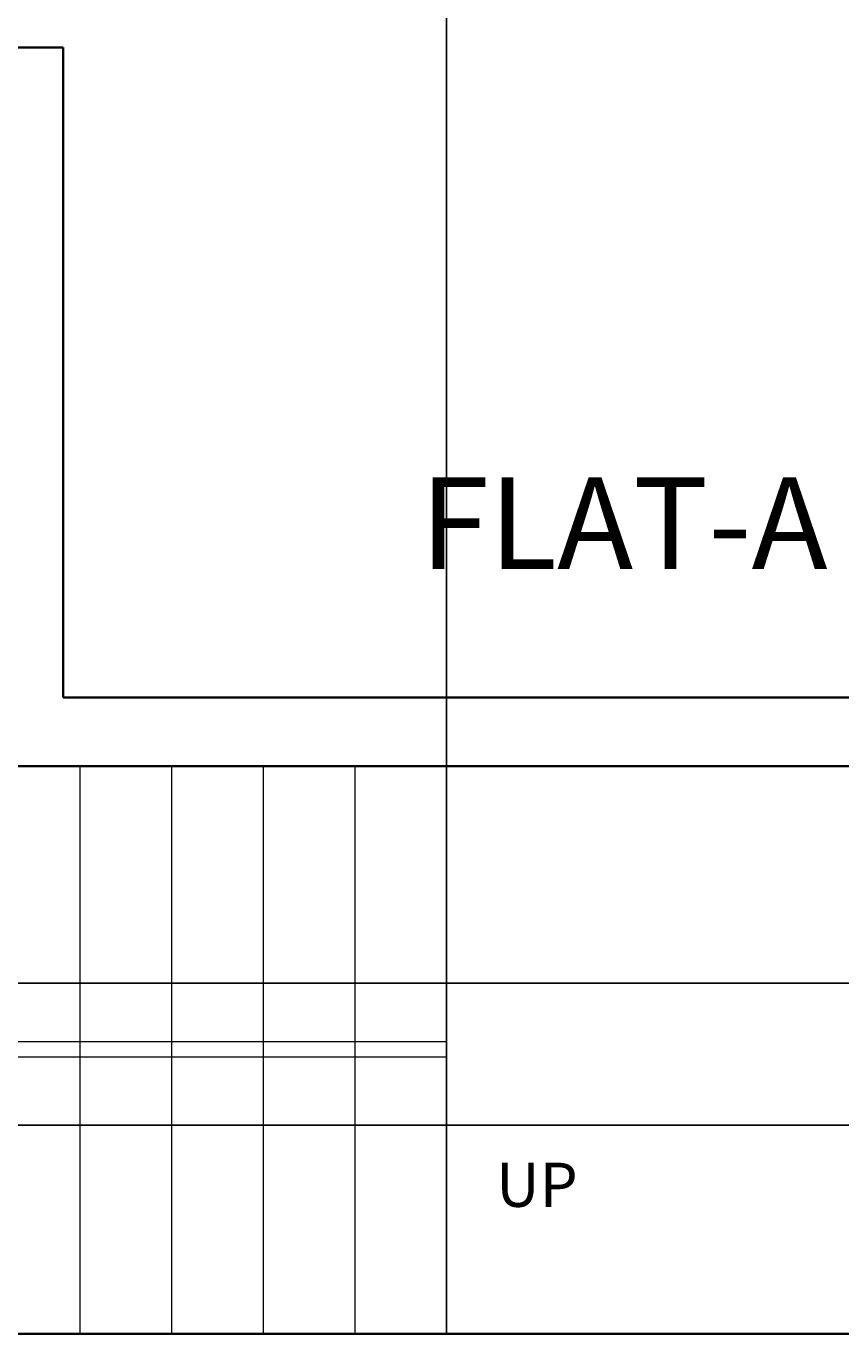
# Model space of a CAD drawing. Units: feet. Extents: x 5816 to 6644, y 25475 to 26788.
# Tile 6 of 23: x 6052 to 6159, y 26094 to 26265. Entities that reach past the tile are written whole.
import ezdxf

# ---------------------------------------------------------------- set-up
doc = ezdxf.new("R2010")
doc.units = ezdxf.units.FT
for name, color, linetype, lineweight in [('A-ANNO-DIMS', 2, 'Continuous', 13), ('A-ANNO-TEXT', 7, 'Continuous', 18), ('A-AREA-IDEN', 7, 'Continuous', 18), ('A-FLOR-STRS', 7, 'Continuous', 18), ('A-WALL', 7, 'Continuous', 35)]:
    doc.layers.add(name, color=color, linetype=linetype, lineweight=lineweight)
doc.styles.get("Standard").update_dxf_attribs({"font": 'arial.ttf'})
doc.dimstyles.get("Standard").update_dxf_attribs({"dimtxt": 0.18, "dimasz": 0.18, "dimexe": 0.18, "dimexo": 0.0625, "dimgap": 0.09, "dimtad": 0, "dimtih": 1, "dimtoh": 1, "dimdec": 4, "dimzin": 0, "dimdsep": 46, "dimtxsty": 'Standard', "dimcen": 0.09, "dimadec": 0, "dimazin": 0, "dimtfac": 1, "dimtdec": 4, "dimtofl": 0, "dimtmove": 0, "dimatfit": 3, "dimfxl": 1, "dimtolj": 1, "dimtzin": 0, "dimarcsym": 0})

# ---------------------------------------------------------------- blocks, each defined once
blk = doc.blocks.new('*D58')
at = {"layer": 'A-ANNO-DIMS', "color": 0, "lineweight": -2, "transparency": 16777216}
for p, q in [((5953.98, 26168.65), (5953.98, 26787.91)), ((5954.16, 26787.73), (6030.2, 26787.73)), ((6106.8, 26787.73), (6030.76, 26787.73)), ((6106.98, 26168.71), (6106.98, 26787.91))]:
    blk.add_line(p, q, dxfattribs=at)
at = {"layer": 'A-ANNO-DIMS', "color": 0, "transparency": 16777216}
for points in [[(5954.16, 26787.76), (5954.16, 26787.7), (5953.98, 26787.73)], [(6106.8, 26787.76), (6106.8, 26787.7), (6106.98, 26787.73)]]:
    blk.add_solid(points, dxfattribs=at)
at = {"layer": 'Defpoints', "color": 0, "transparency": 16777216}
for p in [(6106.98, 26787.73), (5953.98, 26168.58), (6106.98, 26168.65)]:
    blk.add_point(p, dxfattribs=at)
at = {"layer": 'A-ANNO-DIMS', "color": 0, "transparency": 16777216, "insert": (6030.48, 26787.73), "char_height": 0.18, "attachment_point": 5}
blk.add_mtext('\\A1;153', dxfattribs=at)
blk = doc.blocks.new('*D60')
at = {"layer": 'A-ANNO-DIMS', "color": 0, "lineweight": -2, "transparency": 16777216}
for p, q in [((6106.98, 26094.4), (6106.98, 26787.91)), ((6107.16, 26787.73), (6224.93, 26787.73)), ((6343.5, 26787.73), (6225.72, 26787.73)), ((6343.68, 26094.4), (6343.68, 26787.91))]:
    blk.add_line(p, q, dxfattribs=at)
at = {"layer": 'A-ANNO-DIMS', "color": 0, "transparency": 16777216}
for points in [[(6107.16, 26787.76), (6107.16, 26787.7), (6106.98, 26787.73)], [(6343.5, 26787.76), (6343.5, 26787.7), (6343.68, 26787.73)]]:
    blk.add_solid(points, dxfattribs=at)
at = {"layer": 'Defpoints', "color": 0, "transparency": 16777216}
for p in [(6343.68, 26787.73), (6106.98, 26094.34), (6343.68, 26094.34)]:
    blk.add_point(p, dxfattribs=at)
at = {"layer": 'A-ANNO-DIMS', "color": 0, "transparency": 16777216, "insert": (6225.33, 26787.73), "char_height": 0.18, "attachment_point": 5}
blk.add_mtext('\\A1;236.7', dxfattribs=at)
blk = doc.blocks.new('*D71')
at = {"layer": 'A-ANNO-DIMS', "color": 0, "lineweight": -2, "transparency": 16777216}
for p, q in [((6343.61, 26140.22), (5815.98, 26140.22)), ((5816.16, 26140.04), (5816.16, 26131.1)), ((5816.16, 26121.79), (5816.16, 26130.74)), ((6343.61, 26121.61), (5815.98, 26121.61))]:
    blk.add_line(p, q, dxfattribs=at)
at = {"layer": 'A-ANNO-DIMS', "color": 0, "transparency": 16777216}
for points in [[(5816.13, 26140.04), (5816.19, 26140.04), (5816.16, 26140.22)], [(5816.13, 26121.79), (5816.19, 26121.79), (5816.16, 26121.61)]]:
    blk.add_solid(points, dxfattribs=at)
at = {"layer": 'Defpoints', "color": 0, "transparency": 16777216}
for p in [(6343.68, 26140.22), (5816.16, 26121.61), (6343.68, 26121.61)]:
    blk.add_point(p, dxfattribs=at)
at = {"layer": 'A-ANNO-DIMS', "color": 0, "transparency": 16777216, "insert": (5816.16, 26130.92), "char_height": 0.18, "attachment_point": 5}
blk.add_mtext('\\A1;18.61', dxfattribs=at)

msp = doc.modelspace()

# ---------------------------------------------------------------- linework, layer by layer
at = {"layer": 'A-FLOR-STRS'}
for p, q in [((6058.9781, 26168.6509), (6058.9781, 26094.3368)), ((6070.9781, 26168.6509), (6070.9781, 26094.3368)), ((6082.9781, 26168.6509), (6082.9781, 26094.3368)), ((6094.9781, 26168.6509), (6094.9781, 26094.3368)), ((6106.9781, 26168.6509), (6106.9781, 26094.3368)), ((5998.9781, 26132.5846), (6106.9781, 26132.5846)), ((5998.9781, 26130.5846), (6106.9781, 26130.5846))]:
    msp.add_line(p, q, dxfattribs=at)
at = {"layer": 'A-WALL'}
for p, q in [((6042.532, 26262.5846), (6056.8119, 26262.5846)), ((6056.8119, 26253.5846), (6056.8119, 26262.5846)), ((6056.8119, 26177.5846), (6056.8119, 26253.5846)), ((6056.8119, 26177.5846), (6175.0829, 26177.5846)), ((5962.9781, 26168.5846), (6175.0829, 26168.5846)), ((5962.9781, 26094.3368), (6175.0829, 26094.3368))]:
    msp.add_line(p, q, dxfattribs=at)

# ---------------------------------------------------------------- texts
at = {"layer": 'A-ANNO-TEXT'}
msp.add_text('UP', height=5.7752, dxfattribs=at).set_placement((6113.4653, 26110.9454))
at = {"layer": 'A-AREA-IDEN'}
msp.add_text('FLAT-A', height=12, dxfattribs=at).set_placement((6103.5031, 26194.3534))

# ---------------------------------------------------------------- dimensions: what is measured, and where the dimension line sits
at = {"layer": 'A-ANNO-DIMS'}
for base, p1, p2, override, picture, middle in [((6106.9781, 26787.7346), (5953.9781, 26168.5846), (6106.9781, 26168.6509), {"dimdec": 0, "dimlfac": 1, "dimrnd": 0, "dimzin": 0, "dimdsep": 46, "dimlunit": 2}, '*D58', (6030.4781, 26787.7346)), ((6343.6763, 26787.7346), (6106.9781, 26094.3368), (6343.6763, 26094.3368), {"dimdec": 1, "dimlfac": 1, "dimrnd": 0, "dimzin": 0, "dimdsep": 46, "dimlunit": 2}, '*D60', (6225.3272, 26787.7346))]:
    dim = msp.add_linear_dim(base=base, p1=p1, p2=p2, dimstyle='Standard', override=override, dxfattribs=at)
    dim.commit()
    dim.dimension.update_dxf_attribs({"geometry": picture, "text_midpoint": middle})
dim = msp.add_linear_dim(base=(5816.1619, 26121.6124), p1=(6343.6763, 26140.2241), p2=(6343.6763, 26121.6124), angle=90, dimstyle='Standard', override={"dimdec": 2, "dimlfac": 1, "dimrnd": 0, "dimzin": 0, "dimdsep": 46, "dimlunit": 2}, dxfattribs=at)
dim.commit()
dim.dimension.update_dxf_attribs({"geometry": '*D71', "text_midpoint": (5816.1619, 26130.9183)})

doc.saveas('drawing.dxf')
